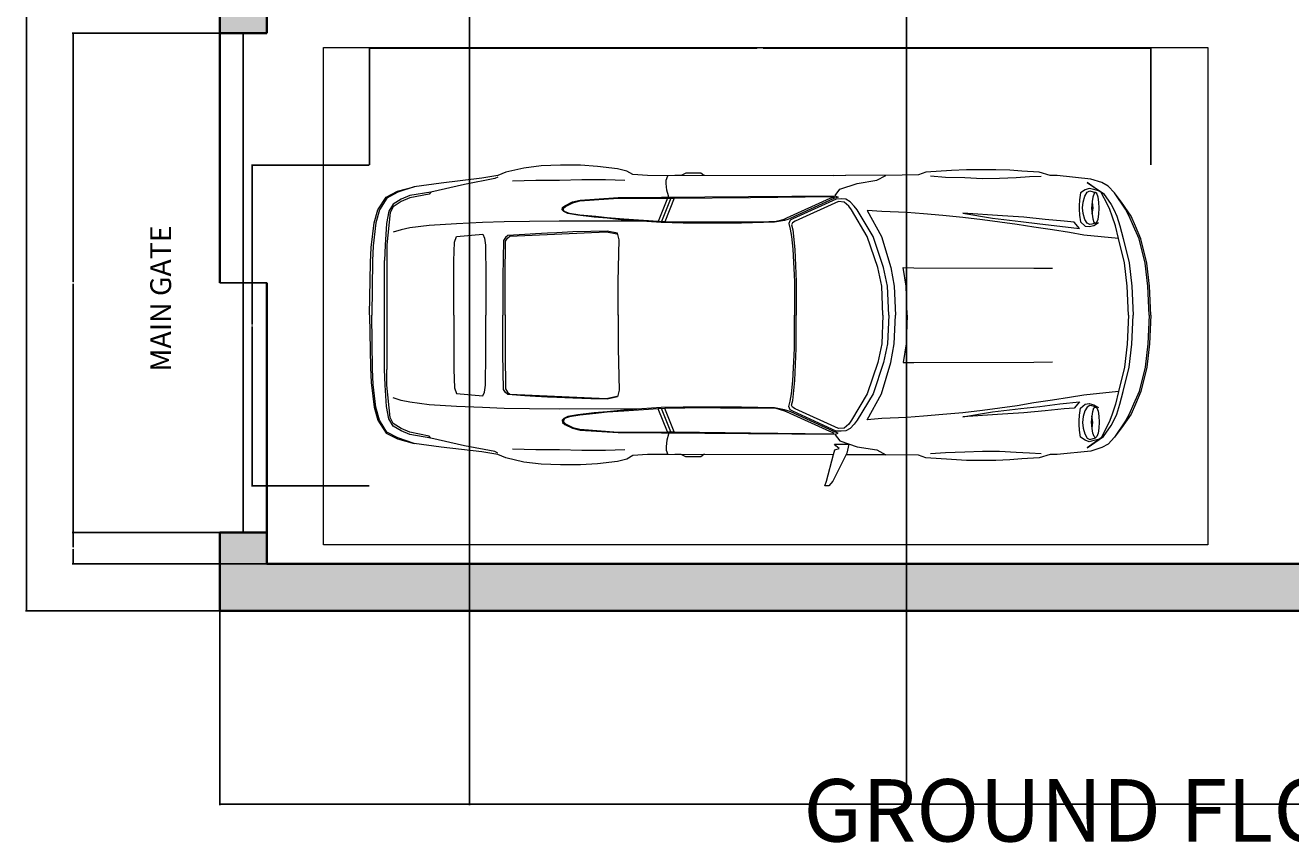
# Model space of a CAD drawing. Units: inches. Extents: x 2701 to 6846, y 811 to 2447.
# Tile 1 of 20: x 2701 to 2944, y 811 to 969. Entities that reach past the tile are written whole.
import ezdxf

# ---------------------------------------------------------------- set-up
doc = ezdxf.new("R2010")
doc.units = ezdxf.units.IN
for name, color, linetype, lineweight in [('A-ANNO-DIMS', 2, 'Continuous', 18), ('A-ANNO-TEXT', 7, 'Continuous', 18), ('A-ANNO-TITL', 7, 'Continuous', 35), ('C-PKNG', 8, 'Continuous', 18), ('C-PKNG-VEHI', 8, 'Continuous', 13), ('C-PROP', 7, 'Continuous', 35), ('C-SITE-GATE', 3, 'Continuous', 25)]:
    doc.layers.add(name, color=color, linetype=linetype, lineweight=lineweight)
doc.layers.add('C-PROP-PATT', color=18, linetype='Continuous', lineweight=13, true_color=0x000000)
doc.styles.get("Standard").update_dxf_attribs({"font": 'arial.ttf'})
doc.dimstyles.get("Standard").update_dxf_attribs({"dimtxt": 0.18, "dimasz": 0.18, "dimexe": 0.18, "dimexo": 0.0625, "dimgap": 0.09, "dimtad": 0, "dimtih": 1, "dimtoh": 1, "dimdec": 4, "dimzin": 0, "dimdsep": 46, "dimtxsty": 'Standard', "dimcen": 0.09, "dimadec": 0, "dimazin": 0, "dimtfac": 1, "dimtdec": 4, "dimtofl": 0, "dimtmove": 0, "dimatfit": 3, "dimfxl": 1, "dimtolj": 1, "dimtzin": 0, "dimarcsym": 0})

# ---------------------------------------------------------------- blocks, each defined once
blk = doc.blocks.new('A$C7AB76BE8')
for p, q in [((1739.9, 1727), (1762, 1752)), ((1762, 1752), (1784, 1752)), ((1784, 1752), (1774.5, 1727)), ((1663.9, 1575), (1739.9, 1727)), ((1774.5, 1727), (1736.1, 1582.3)), ((550.5, 1581.5), (610.5, 1600.1)), ((610.5, 1600.1), (705.5, 1605.7)), ((705.5, 1605.7), (772, 1610.8)), ((772, 1610.8), (847.5, 1613.9)), ((847.5, 1613.9), (920.5, 1613.9)), ((920.5, 1613.9), (1009, 1613.9)), ((1009, 1613.9), (1091.5, 1608.7)), ((1091.5, 1608.7), (1230.5, 1600.1)), ((1230.5, 1600.1), (1271.9, 1585.4)), ((2445.4, 1581.9), (2461.4, 1594.4)), ((2461.4, 1594.4), (2543.4, 1594.4)), ((2543.4, 1594.4), (2568.9, 1581.9)), ((2834.4, 1587.5), (2866.4, 1606.5)), ((2866.4, 1606.5), (2916.9, 1619)), ((2916.9, 1619), (3027.4, 1632)), ((3027.4, 1632), (3119.4, 1638)), ((3119.4, 1638), (3229.9, 1638)), ((3229.9, 1638), (3334.4, 1635)), ((3334.4, 1635), (3429.4, 1622.5)), ((3429.4, 1622.5), (3527.4, 1600.5)), ((3527.4, 1600.5), (3571.8, 1582.3)), ((199, 1486.5), (234, 1524.5)), ((234, 1524.5), (268.5, 1543.5)), ((348.4, 1544.8), (259, 1483.9)), ((268.5, 1543.5), (329, 1562.5)), ((272, 1489.5), (348.4, 1544.8)), ((329, 1562.5), (512.5, 1581.5)), ((512.5, 1581.5), (550.5, 1581.5)), ((601, 1577.2), (664, 1574.1)), ((664, 1574.1), (737, 1569.8)), ((737, 1569.8), (828.5, 1565.5)), ((828.5, 1565.5), (920.5, 1564.6)), ((920.5, 1564.6), (1017.2, 1569)), ((1017.2, 1569), (1123, 1572)), ((1123, 1572), (1206.3, 1578)), ((1271.9, 1585.4), (1448.9, 1582.8)), ((1448.9, 1582.8), (1667.8, 1583.2)), ((1499.5, 1556), (1448.9, 1582.8)), ((1607, 1539.2), (1499.5, 1556)), ((1701.9, 1507.2), (1607, 1539.2)), ((1651.4, 1524.5), (1663.9, 1575)), ((1730.4, 1524.5), (1651.4, 1524.5)), ((1729.6, 1556), (1705, 1549.5)), ((1705, 1549.5), (1723.5, 1534.4)), ((1723.5, 1534.4), (1730.4, 1524.5)), ((1736.1, 1582.3), (1729.6, 1556)), ((1736.1, 1582.8), (2641.4, 1581.1)), ((2438.9, 1581.9), (2445.4, 1581.9)), ((2568.9, 1581.9), (2603.4, 1581.9)), ((2641.4, 1581.1), (2753.2, 1581.5)), ((2650.9, 1557.3), (2641.4, 1581.1)), ((2647.9, 1502.5), (2650.9, 1537.9)), ((2650.9, 1537.9), (2650.9, 1557.3)), ((2753.2, 1581.5), (2834.4, 1587.5)), ((2878, 1555.4), (2982.5, 1558.8)), ((2982.5, 1558.8), (3112, 1558.8)), ((3112, 1558.8), (3235.5, 1555.4)), ((3235.5, 1555.4), (3363.3, 1555.4)), ((3363.3, 1555.4), (3491.5, 1551.9)), ((3571.8, 1582.3), (3660.3, 1566.8)), ((3571.8, 1573.7), (3587.4, 1565.1)), ((3587.4, 1565.1), (3754, 1533.6)), ((3660.3, 1566.8), (3881.8, 1540.9)), ((3754, 1533.6), (3938.8, 1491.7)), ((3881.8, 1540.9), (4030.3, 1521)), ((139, 1398), (199, 1486.5)), ((161, 1435.6), (199, 1486.5)), ((259, 1483.9), (218, 1423.5)), ((237, 1423.5), (272, 1489.5)), ((284.1, 1436.9), (288.8, 1464.5)), ((287.5, 1499), (313, 1505.5)), ((288.8, 1464.5), (295.3, 1483)), ((295.3, 1483), (303.5, 1489.5)), ((333.3, 1498.6), (303.5, 1489.5)), ((303.5, 1489.5), (310.9, 1483)), ((310.9, 1483), (317.8, 1464.5)), ((313, 1505.5), (338.5, 1511.5)), ((317.8, 1464.5), (322.1, 1439.4)), ((349.3, 1491.3), (333.3, 1498.6)), ((338.5, 1511.5), (359.6, 1503.8)), ((361.8, 1469.2), (349.3, 1491.3)), ((359.6, 1503.8), (384.7, 1486.5)), ((370.4, 1437.3), (361.8, 1469.2)), ((384.7, 1486.5), (391.2, 1448.5)), ((1668.7, 1452), (1693.7, 1454.1)), ((1693.7, 1454.1), (1720.9, 1453.3)), ((1727.4, 1473.1), (1701.9, 1507.2)), ((1727.4, 1470.5), (1709.7, 1464.1)), ((1709.7, 1464.1), (1734.3, 1455.8)), ((2913.9, 1461.5), (1727.4, 1470.5)), ((1741.2, 1467.5), (1731.7, 1464.1)), ((1731.7, 1464.1), (1756.8, 1455.8)), ((1734.3, 1455.8), (1970.1, 1348.3)), ((2189.8, 1462.8), (1741.2, 1467.5)), ((1756.8, 1455.8), (1992.5, 1348.3)), ((2606.9, 1458), (2189.8, 1462.8)), ((2638.4, 1458), (2606.9, 1458)), ((2606.9, 1458), (2658.3, 1329.8)), ((2625.4, 1458), (2676.8, 1330.6)), ((2638.4, 1470.5), (2647.9, 1502.5)), ((2638.4, 1458), (2638.4, 1470.5)), ((2913.9, 1458.4), (2638.4, 1458)), ((2644, 1458), (2695, 1331.5)), ((3122.4, 1447.6), (2913.9, 1461.5)), ((3122.8, 1443.8), (2913.9, 1458.4)), ((3938.8, 1491.7), (4052.8, 1472.3)), ((3938.8, 1491.7), (3948.3, 1480.9)), ((3948.3, 1480.9), (4052.8, 1459.3)), ((4120.8, 1496.3), (4030.3, 1521)), ((4030.3, 1521), (4118.9, 1490.4)), ((4052.8, 1472.3), (4099.9, 1452.8)), ((4052.8, 1459.3), (4099.9, 1439.9)), ((4118.9, 1490.4), (4178.4, 1458.4)), ((4182.3, 1464.5), (4120.8, 1496.3)), ((4178.4, 1458.4), (4219, 1394.5)), ((4228.5, 1394.5), (4182.3, 1464.5)), ((108.8, 1360), (161, 1435.6)), ((118.3, 1360), (139, 1398)), ((202.1, 1395.4), (186.5, 1360.4)), ((218, 1423.5), (202.1, 1395.4)), ((211.6, 1360.4), (224.5, 1395.4)), ((224.5, 1395.4), (237, 1423.5)), ((282.8, 1404), (284.1, 1436.9)), ((284.1, 1371.7), (282.8, 1404)), ((321.2, 1436.9), (316.9, 1404)), ((316.9, 1404), (322.5, 1372.1)), ((324.2, 1404), (321.2, 1371.7)), ((322.1, 1439.4), (324.2, 1404)), ((373.5, 1405.8), (370.4, 1437.3)), ((370.4, 1374.2), (373.5, 1405.8)), ((391.2, 1448.5), (392.5, 1417)), ((392.5, 1398), (391.2, 1366)), ((392.5, 1417), (392.5, 1398)), ((1335, 1379), (1471.8, 1385)), ((1471.8, 1385), (1551.7, 1391.5)), ((1551.7, 1391.5), (1473.1, 1249.5)), ((1519.3, 1249.5), (1607, 1394.5)), ((1551.3, 1249.5), (1637.6, 1394.5)), ((1607, 1394.5), (1622.1, 1415.3)), ((1622.1, 1415.3), (1645, 1439)), ((1637.6, 1394.5), (1651.4, 1415.3)), ((1645, 1439), (1668.7, 1452)), ((1651.4, 1415.3), (1676.9, 1437.3)), ((1676.9, 1437.3), (1709.3, 1439.4)), ((1709.3, 1439.4), (1946.3, 1331.9)), ((1720.9, 1453.3), (1959.3, 1344.9)), ((3163, 1437.7), (3122.4, 1447.6)), ((3161.2, 1433), (3122.8, 1443.8)), ((3201.8, 1413.1), (3161.2, 1433)), ((3206.1, 1416.6), (3163, 1437.7)), ((3179.8, 1375.1), (3207, 1385)), ((3189, 1373.7), (3211.8, 1385)), ((3213.1, 1403.6), (3201.8, 1413.1)), ((3219.1, 1406.6), (3206.1, 1416.6)), ((3207, 1385), (3213.5, 1393.2)), ((3211.8, 1385), (3220.4, 1393.7)), ((3213.5, 1393.2), (3213.1, 1403.6)), ((3220.4, 1393.7), (3219.1, 1406.6)), ((4099.9, 1452.8), (4144.3, 1426.1)), ((4099.9, 1439.9), (4144.3, 1411.4)), ((4144.3, 1426.1), (4168.1, 1386.8)), ((4144.3, 1411.4), (4160.3, 1379)), ((4168.1, 1386.8), (4180.2, 1319.8)), ((4219, 1394.5), (4238.9, 1322.9)), ((4248.4, 1322.9), (4228.5, 1394.5)), ((85.1, 1306), (108.8, 1360)), ((94.6, 1306), (118.3, 1360)), ((186.5, 1360.4), (169.2, 1306.5)), ((194.3, 1306.5), (211.6, 1360.4)), ((288.8, 1343.6), (284.1, 1371.7)), ((313, 1309.1), (287.5, 1325)), ((295.3, 1326.3), (288.8, 1343.6)), ((303.5, 1320.7), (295.3, 1326.3)), ((311.3, 1326.8), (303.5, 1320.7)), ((303.5, 1320.7), (323.8, 1315.5)), ((318.2, 1345.8), (311.3, 1326.8)), ((321.2, 1371.7), (318.2, 1345.8)), ((323.8, 1315.5), (333.3, 1313.8)), ((333.3, 1313.8), (349.3, 1322)), ((349.3, 1322), (361.8, 1342.3)), ((384.7, 1328.1), (359.6, 1305.6)), ((361.8, 1342.3), (370.4, 1374.2)), ((391.2, 1366), (384.7, 1328.1)), ((390.3, 1293.1), (418.8, 1327.6)), ((418.8, 1327.6), (474.9, 1332.4)), ((474.9, 1332.4), (577.7, 1342.3)), ((607, 1318.1), (498.7, 1304.3)), ((577.7, 1342.3), (695.1, 1353.5)), ((711.9, 1330.6), (607, 1318.1)), ((695.1, 1353.5), (812.5, 1361.7)), ((866.5, 1348.8), (711.9, 1330.6)), ((731.4, 1314.7), (920.5, 1340.1)), ((812.5, 1361.7), (1028, 1376)), ((1028, 1376), (866.5, 1348.8)), ((920.5, 1340.1), (1028, 1352.7)), ((1028, 1352.7), (1138.9, 1363)), ((1138.9, 1363), (1243, 1372.5)), ((1243, 1372.5), (1335, 1379)), ((1946.3, 1331.9), (1960.6, 1323.3)), ((1959.3, 1344.9), (1973.5, 1337.5)), ((1960.6, 1323.3), (1966.2, 1311.6)), ((1970.1, 1348.3), (1986, 1342.3)), ((1973.5, 1337.5), (1979.6, 1319)), ((1979.6, 1319), (1973.5, 1289.2)), ((1986, 1342.3), (2003.3, 1336.3)), ((1992.5, 1348.3), (2008.5, 1342.3)), ((2003.3, 1336.3), (2058.1, 1326.3)), ((2008.5, 1342.3), (2025.8, 1336.3)), ((2025.8, 1336.3), (2049.1, 1330.2)), ((2049.1, 1330.2), (2130.7, 1327.6)), ((2058.1, 1326.3), (2239.9, 1322)), ((2130.7, 1327.6), (2239.5, 1327.6)), ((2239.5, 1327.6), (2354.7, 1327.2)), ((2239.9, 1322), (2438.9, 1322)), ((2354.7, 1327.2), (2439.4, 1326.3)), ((2438.9, 1322), (2558.1, 1322)), ((2439.4, 1326.3), (2658.3, 1329.8)), ((2558.1, 1322), (2679, 1325.2)), ((2658.3, 1329.8), (2695.4, 1331.5)), ((2679, 1325.2), (2783.9, 1332.4)), ((2695.4, 1331.5), (2881.9, 1344)), ((2783.9, 1332.4), (2881.9, 1338.8)), ((2783.9, 1332.4), (3236.4, 1333.2)), ((2881.9, 1344), (2973.9, 1350.5)), ((2881.9, 1338.8), (2973.2, 1348.1)), ((2973.2, 1348.1), (3044.4, 1354.2)), ((2973.9, 1350.5), (3036, 1357.4)), ((3036, 1357.4), (3123.2, 1366)), ((3044.4, 1354.2), (3135.1, 1364.6)), ((3123.2, 1366), (3179.8, 1375.1)), ((3135.1, 1364.6), (3189, 1373.7)), ((3236.4, 1333.2), (3397.8, 1331.5)), ((3397.8, 1331.5), (3536.9, 1329.8)), ((3536.9, 1329.8), (3655.2, 1324.6)), ((3655.2, 1324.6), (3797.2, 1318.1)), ((3797.2, 1318.1), (3948.3, 1309.5)), ((4160.3, 1379), (4178.3, 1202.8)), ((4180.2, 1319.8), (4187.9, 1201.5)), ((4238.9, 1322.9), (4254.4, 1198.1)), ((4264.8, 1188.6), (4248.4, 1322.9)), ((55.3, 1236.5), (85.1, 1306)), ((64.8, 1236.5), (94.6, 1306)), ((169.2, 1306.5), (151.5, 1237)), ((177, 1237), (194.3, 1306.5)), ((177, 1237), (366.1, 1256.8)), ((338.5, 1303), (313, 1309.1)), ((359.6, 1305.6), (338.5, 1303)), ((366.1, 1256.8), (444.3, 1269.8)), ((498.7, 1304.3), (390.3, 1293.1)), ((444.3, 1269.8), (538, 1284.4)), ((538, 1284.4), (639.8, 1299.6)), ((639.8, 1299.6), (731.4, 1314.7)), ((1473.1, 1249.5), (1422.6, 1078.5)), ((1462.3, 1078.5), (1519.3, 1249.5)), ((1494.3, 1078.5), (1551.3, 1249.5)), ((1958.8, 1285.7), (1947.6, 1177.4)), ((1965.7, 1249.5), (1957.5, 1179.5)), ((1966.2, 1311.6), (1958.8, 1285.7)), ((1973.5, 1289.2), (1965.7, 1249.5)), ((2907.4, 1230.5), (2916.9, 1266.7)), ((2916.9, 1266.7), (2973.4, 1278.4)), ((2977.8, 1274.9), (2921.2, 1263.3)), ((2973.4, 1278.4), (3064.1, 1276.7)), ((3505.8, 1250.8), (2977.8, 1274.9)), ((3064.1, 1276.7), (3162.5, 1273.7)), ((3162.5, 1273.7), (3249.8, 1269.3)), ((3249.8, 1269.3), (3300.3, 1267.6)), ((3300.3, 1267.6), (3365.5, 1263.7)), ((3365.5, 1263.7), (3423.3, 1260.3)), ((3423.3, 1260.3), (3516.6, 1254.2)), ((3519.2, 1240), (3505.8, 1250.8)), ((3516.6, 1254.2), (3530, 1243)), ((3654.7, 1260.7), (3645.2, 1240.4)), ((3797.6, 1248.2), (3654.7, 1260.7)), ((3809.7, 1217.5), (3797.6, 1248.2)), ((3948.3, 1309.5), (4052.8, 1296.1)), ((4052.8, 1296.1), (4099.9, 1285.3)), ((4099.9, 1285.3), (4144.3, 1272.4)), ((22, 1103.5), (55.3, 1236.5)), ((31.5, 1103.5), (64.8, 1236.5)), ((151.5, 1237), (118.3, 1104)), ((143.8, 1104), (177, 1237)), ((1947.6, 1177.4), (1940.7, 1002.1)), ((1957.5, 1179.5), (1948.5, 1002.1)), ((2913.4, 1002.5), (2907.4, 1230.5)), ((3529.1, 1222.7), (3519.2, 1240)), ((3531.2, 1027.6), (3529.1, 1222.7)), ((3530, 1243), (3540.3, 1226.2)), ((3540.3, 1226.2), (3543.8, 1030.6)), ((3638.8, 1202), (3637.9, 1030.6)), ((3645.2, 1240.4), (3638.8, 1202)), ((3813.2, 1116.1), (3809.7, 1217.5)), ((4178.3, 1202.8), (4179.5, 1117.3)), ((4187.9, 1201.5), (4191, 1116.5)), ((4254.4, 1198.1), (4257.9, 1115.6)), ((4268.2, 1106.1), (4264.8, 1188.6)), ((3813.2, 819), (3813.2, 1116.1)), ((4179.5, 520.7), (4179.5, 1117.3)), ((4191, 1116.5), (4191, 521.5)), ((4257.9, 1115.6), (4261.3, 819)), ((7.8, 977), (22, 1103.5)), ((17.3, 977), (31.5, 1103.5)), ((118.3, 1104), (104.1, 977.5)), ((129.5, 977.5), (143.8, 1104)), ((639.8, 1075.9), (538, 1074.6)), ((1296.5, 1078.1), (639.8, 1075.9)), ((1354.4, 1078.5), (1296.5, 1078.1)), ((1338.8, 977), (1354.4, 1078.5)), ((1422.6, 1078.5), (1403.6, 977)), ((1440.3, 977), (1462.3, 1078.5)), ((1472.3, 977), (1494.3, 1078.5)), ((4273.9, 819.5), (4268.2, 1106.1)), ((0, 819), (7.8, 977)), ((9.1, 819), (17.3, 977)), ((104.1, 977.5), (96.3, 819)), ((121.8, 819), (129.5, 977.5)), ((1332.4, 819), (1338.8, 977)), ((1403.6, 977), (1397.1, 819)), ((1433.8, 819), (1440.3, 977)), ((1465.8, 819), (1472.3, 977)), ((1940.7, 1002.1), (1939.4, 819)), ((1948.5, 1002.1), (1949.3, 819)), ((2913.9, 818.6), (2913.4, 1002.5)), ((3531.2, 818.6), (3531.2, 1027.6)), ((3543.8, 1030.6), (3543.8, 819)), ((3637.9, 1030.6), (3637.9, 819)), ((0, 819), (7.8, 661)), ((9.1, 819), (17.3, 661)), ((104.1, 660.6), (96.3, 819)), ((121.8, 819), (129.5, 660.6)), ((1332.4, 819), (1338.8, 661)), ((1403.6, 661), (1397.1, 819)), ((1433.8, 819), (1440.3, 661)), ((1465.8, 819), (1472.3, 661)), ((1940.7, 636), (1939.4, 819)), ((1948.5, 636), (1949.3, 819)), ((2913.9, 819.5), (2913.4, 635.5)), ((3531.2, 819.5), (3531.2, 610.5)), ((3543.8, 607.5), (3543.8, 819)), ((3637.9, 607.5), (3637.9, 819)), ((3813.2, 819), (3813.2, 522)), ((4257.9, 522.4), (4261.3, 819)), ((4273.9, 818.6), (4268.2, 531.9)), ((7.8, 661), (22, 534.5)), ((17.3, 661), (31.5, 534.5)), ((118.3, 534.1), (104.1, 660.6)), ((129.5, 660.6), (143.8, 534.1)), ((1338.8, 661), (1354.4, 559.5)), ((1422.6, 559.5), (1403.6, 661)), ((1440.3, 661), (1462.3, 559.5)), ((1472.3, 661), (1494.3, 559.5)), ((1947.6, 460.7), (1940.7, 636)), ((1957.5, 458.5), (1948.5, 636)), ((2913.4, 635.5), (2907.4, 407.6)), ((639.8, 562.1), (538, 563.4)), ((1296.5, 560), (639.8, 562.1)), ((1354.4, 559.5), (1296.5, 560)), ((1473.1, 388.6), (1422.6, 559.5)), ((1462.3, 559.5), (1519.3, 388.6)), ((1494.3, 559.5), (1551.3, 388.6)), ((3531.2, 610.5), (3529.1, 415.3)), ((3540.3, 411.9), (3543.8, 607.5)), ((3638.8, 436.1), (3637.9, 607.5)), ((22, 534.5), (55.3, 401.5)), ((31.5, 534.5), (64.8, 401.5)), ((151.5, 401.1), (118.3, 534.1)), ((143.8, 534.1), (177, 401.1)), ((3813.2, 522), (3809.7, 420.5)), ((4178.3, 435.3), (4179.5, 520.7)), ((4187.9, 436.5), (4191, 521.5)), ((4254.4, 439.9), (4257.9, 522.4)), ((4268.2, 531.9), (4264.8, 449.4)), ((1958.8, 352.3), (1947.6, 460.7)), ((1965.7, 388.6), (1957.5, 458.5)), ((3529.1, 415.3), (3519.2, 398.1)), ((3645.2, 397.6), (3638.8, 436.1)), ((3809.7, 420.5), (3797.6, 389.9)), ((4160.3, 259), (4178.3, 435.3)), ((4180.2, 318.2), (4187.9, 436.5)), ((4238.9, 315.2), (4254.4, 439.9)), ((4264.8, 449.4), (4248.4, 315.2)), ((55.3, 401.5), (85.1, 332)), ((64.8, 401.5), (94.6, 332)), ((169.2, 331.6), (151.5, 401.1)), ((177, 401.1), (194.3, 331.6)), ((177, 401.1), (366.1, 381.2)), ((366.1, 381.2), (444.3, 368.3)), ((444.3, 368.3), (538, 353.6)), ((538, 353.6), (639.8, 338.5)), ((1551.7, 246.5), (1473.1, 388.6)), ((1519.3, 388.6), (1607, 243.5)), ((1551.3, 388.6), (1637.6, 243.5)), ((1966.2, 326.4), (1958.8, 352.3)), ((1973.5, 348.9), (1965.7, 388.6)), ((1979.6, 319.1), (1973.5, 348.9)), ((2907.4, 407.6), (2916.9, 371.3)), ((2916.9, 371.3), (2973.4, 359.6)), ((2977.8, 363.1), (2921.2, 374.8)), ((2973.4, 359.6), (3064.1, 361.4)), ((3505.8, 387.3), (2977.8, 363.1)), ((3064.1, 361.4), (3162.5, 364.4)), ((3162.5, 364.4), (3249.8, 368.7)), ((3249.8, 368.7), (3300.3, 370.4)), ((3300.3, 370.4), (3365.5, 374.3)), ((3365.5, 374.3), (3423.3, 377.8)), ((3423.3, 377.8), (3516.6, 383.8)), ((3519.2, 398.1), (3505.8, 387.3)), ((3516.6, 383.8), (3530, 395)), ((3530, 395), (3540.3, 411.9)), ((3654.7, 377.3), (3645.2, 397.6)), ((3797.6, 389.9), (3654.7, 377.3)), ((4052.8, 341.9), (4099.9, 352.7)), ((4099.9, 352.7), (4144.3, 365.7)), ((85.1, 332), (108.8, 278)), ((94.6, 332), (118.3, 278)), ((108.8, 278), (161, 202.5)), ((118.3, 278), (139, 240.1)), ((186.5, 277.6), (169.2, 331.6)), ((202.1, 242.6), (186.5, 277.6)), ((194.3, 331.6), (211.6, 277.6)), ((211.6, 277.6), (224.5, 242.6)), ((288.8, 294.5), (284.1, 266.4)), ((313, 329), (287.5, 313)), ((295.3, 311.7), (288.8, 294.5)), ((303.5, 317.3), (295.3, 311.7)), ((303.5, 317.3), (323.8, 322.5)), ((311.3, 311.3), (303.5, 317.3)), ((318.2, 292.3), (311.3, 311.3)), ((338.5, 335), (313, 329)), ((321.2, 266.4), (318.2, 292.3)), ((323.8, 322.5), (333.3, 324.2)), ((333.3, 324.2), (349.3, 316)), ((359.6, 332.4), (338.5, 335)), ((349.3, 316), (361.8, 295.7)), ((384.7, 310), (359.6, 332.4)), ((361.8, 295.7), (370.4, 263.8)), ((391.2, 272), (384.7, 310)), ((390.3, 345), (418.8, 310.4)), ((498.7, 333.7), (390.3, 345)), ((418.8, 310.4), (474.9, 305.7)), ((474.9, 305.7), (577.7, 295.7)), ((607, 319.9), (498.7, 333.7)), ((577.7, 295.7), (695.1, 284.5)), ((711.9, 307.4), (607, 319.9)), ((639.8, 338.5), (731.4, 323.4)), ((695.1, 284.5), (812.5, 276.3)), ((866.5, 289.3), (711.9, 307.4)), ((731.4, 323.4), (920.5, 297.9)), ((1028, 262.1), (866.5, 289.3)), ((920.5, 297.9), (1028, 285.4)), ((1028, 285.4), (1138.9, 275)), ((1709.3, 198.6), (1946.3, 306.1)), ((1720.9, 184.8), (1959.3, 293.2)), ((1734.3, 182.2), (1970.1, 289.7)), ((1756.8, 182.2), (1992.5, 289.7)), ((1946.3, 306.1), (1960.6, 314.7)), ((1959.3, 293.2), (1973.5, 300.5)), ((1960.6, 314.7), (1966.2, 326.4)), ((1970.1, 289.7), (1986, 295.7)), ((1973.5, 300.5), (1979.6, 319.1)), ((1986, 295.7), (2003.3, 301.8)), ((1992.5, 289.7), (2008.5, 295.7)), ((2003.3, 301.8), (2058.1, 311.7)), ((2008.5, 295.7), (2025.8, 301.8)), ((2025.8, 301.8), (2049.1, 307.8)), ((2049.1, 307.8), (2130.7, 310.4)), ((2058.1, 311.7), (2239.9, 316)), ((2130.7, 310.4), (2239.5, 310.4)), ((2239.5, 310.4), (2354.7, 310.9)), ((2239.9, 316), (2438.9, 316)), ((2354.7, 310.9), (2439.4, 311.7)), ((2438.9, 316), (2558.1, 316)), ((2439.4, 311.7), (2658.3, 308.3)), ((2558.1, 316), (2679, 312.8)), ((2606.9, 180), (2658.3, 308.3)), ((2625.4, 180), (2676.8, 307.4)), ((2644, 180), (2695, 306.5)), ((2658.3, 308.3), (2695.4, 306.5)), ((2679, 312.8), (2783.9, 305.7)), ((2695.4, 306.5), (2881.9, 294)), ((2783.9, 305.7), (3236.4, 304.8)), ((2783.9, 305.7), (2881.9, 299.2)), ((2881.9, 299.2), (2973.2, 290)), ((2881.9, 294), (2973.9, 287.5)), ((2973.2, 290), (3044.4, 283.9)), ((2973.9, 287.5), (3036, 280.6)), ((3036, 280.6), (3123.2, 272)), ((3044.4, 283.9), (3135.1, 273.4)), ((3236.4, 304.8), (3397.8, 306.5)), ((3397.8, 306.5), (3536.9, 308.3)), ((3536.9, 308.3), (3655.2, 313.4)), ((3655.2, 313.4), (3797.2, 319.9)), ((3797.2, 319.9), (3948.3, 328.6)), ((3948.3, 328.6), (4052.8, 341.9)), ((4168.1, 251.3), (4180.2, 318.2)), ((4219, 243.5), (4238.9, 315.2)), ((4248.4, 315.2), (4228.5, 243.5)), ((139, 240.1), (199, 151.5)), ((218, 214.6), (202.1, 242.6)), ((259, 154.1), (218, 214.6)), ((224.5, 242.6), (237, 214.6)), ((237, 214.6), (272, 148.5)), ((284.1, 266.4), (282.8, 234)), ((282.8, 234), (284.1, 201.2)), ((316.9, 234), (322.5, 266)), ((321.2, 201.2), (316.9, 234)), ((324.2, 234), (321.2, 266.4)), ((322.1, 198.6), (324.2, 234)), ((370.4, 263.8), (373.5, 232.3)), ((373.5, 232.3), (370.4, 200.8)), ((392.5, 240.1), (391.2, 272)), ((391.2, 189.5), (392.5, 221.1)), ((392.5, 221.1), (392.5, 240.1)), ((812.5, 276.3), (1028, 262.1)), ((1138.9, 275), (1243, 265.5)), ((1243, 265.5), (1335, 259)), ((1335, 259), (1471.8, 253)), ((1471.8, 253), (1551.7, 246.5)), ((1607, 243.5), (1622.1, 222.8)), ((1622.1, 222.8), (1645, 199)), ((1637.6, 243.5), (1651.4, 222.8)), ((1651.4, 222.8), (1676.9, 200.8)), ((3123.2, 272), (3179.8, 262.9)), ((3135.1, 273.4), (3189, 264.3)), ((3201.8, 224.9), (3161.2, 205.1)), ((3206.1, 221.5), (3163, 200.3)), ((3179.8, 262.9), (3207, 253)), ((3189, 264.3), (3211.8, 253)), ((3213.1, 234.4), (3201.8, 224.9)), ((3219.1, 231.4), (3206.1, 221.5)), ((3207, 253), (3213.5, 244.8)), ((3211.8, 253), (3220.4, 244.4)), ((3213.5, 244.8), (3213.1, 234.4)), ((3220.4, 244.4), (3219.1, 231.4)), ((4099.9, 198.2), (4144.3, 226.7)), ((4099.9, 185.2), (4144.3, 212)), ((4144.3, 226.7), (4160.3, 259)), ((4144.3, 212), (4168.1, 251.3)), ((4178.4, 179.6), (4219, 243.5)), ((4228.5, 243.5), (4182.3, 173.6)), ((161, 202.5), (199, 151.5)), ((199, 151.5), (234, 113.5)), ((348.4, 93.3), (259, 154.1)), ((272, 148.5), (348.4, 93.3)), ((284.1, 201.2), (288.8, 173.6)), ((287.5, 139), (313, 132.5)), ((288.8, 173.6), (295.3, 155)), ((295.3, 155), (303.5, 148.5)), ((303.5, 148.5), (310.9, 155)), ((333.3, 139.5), (303.5, 148.5)), ((310.9, 155), (317.8, 173.6)), ((317.8, 173.6), (322.1, 198.6)), ((349.3, 146.8), (333.3, 139.5)), ((361.8, 168.8), (349.3, 146.8)), ((359.6, 134.3), (384.7, 151.5)), ((370.4, 200.8), (361.8, 168.8)), ((384.7, 151.5), (391.2, 189.5)), ((1645, 199), (1668.7, 186.1)), ((1668.7, 186.1), (1693.7, 183.9)), ((1676.9, 200.8), (1709.3, 198.6)), ((1693.7, 183.9), (1720.9, 184.8)), ((1727.4, 164.9), (1701.9, 130.8)), ((1709.7, 174), (1734.3, 182.2)), ((1727.4, 167.5), (1709.7, 174)), ((2913.9, 176.6), (1727.4, 167.5)), ((1731.7, 174), (1756.8, 182.2)), ((1741.2, 170.5), (1731.7, 174)), ((2189.8, 175.3), (1741.2, 170.5)), ((2606.9, 180), (2189.8, 175.3)), ((2638.4, 180), (2606.9, 180)), ((2638.4, 180), (2638.4, 167.5)), ((2913.9, 179.6), (2638.4, 180)), ((2638.4, 167.5), (2647.9, 135.6)), ((3122.8, 194.3), (2913.9, 179.6)), ((3122.4, 190.4), (2913.9, 176.6)), ((3163, 200.3), (3122.4, 190.4)), ((3161.2, 205.1), (3122.8, 194.3)), ((3754, 104.5), (3938.8, 146.4)), ((3938.8, 146.4), (4052.8, 165.8)), ((3938.8, 146.4), (3948.3, 157.2)), ((3948.3, 157.2), (4052.8, 178.7)), ((4030.3, 117), (4118.9, 147.7)), ((4120.8, 141.8), (4030.3, 117)), ((4052.8, 178.7), (4099.9, 198.2)), ((4052.8, 165.8), (4099.9, 185.2)), ((4118.9, 147.7), (4178.4, 179.6)), ((4182.3, 173.6), (4120.8, 141.8)), ((234, 113.5), (268.5, 94.6)), ((268.5, 94.6), (329, 75.6)), ((313, 132.5), (338.5, 126.5)), ((329, 75.6), (512.5, 56.6)), ((338.5, 126.5), (359.6, 134.3)), ((737, 68.2), (828.5, 72.5)), ((828.5, 72.5), (920.5, 73.4)), ((920.5, 73.4), (1017.2, 69.1)), ((1499.5, 82), (1448.9, 55.3)), ((1607, 98.9), (1499.5, 82)), ((1701.9, 130.8), (1607, 98.9)), ((2650.9, 80.7), (2641.4, 57)), ((2647.9, 135.6), (2650.9, 100.2)), ((2650.9, 100.2), (2650.9, 80.7)), ((2878, 82.7), (2982.5, 79.2)), ((2982.5, 79.2), (3112, 79.2)), ((3112, 79.2), (3235.5, 82.7)), ((3235.5, 82.7), (3363.3, 82.7)), ((3363.3, 82.7), (3491.5, 86.1)), ((3571.8, 64.3), (3587.4, 73)), ((3571.8, 55.7), (3660.3, 71.2)), ((3587.4, 73), (3754, 104.5)), ((3660.3, 71.2), (3881.8, 97.1)), ((3881.8, 97.1), (4030.3, 117)), ((512.5, 56.6), (550.5, 56.6)), ((550.5, 56.6), (610.5, 38)), ((601, 60.9), (664, 63.9)), ((610.5, 38), (705.5, 32.4)), ((664, 63.9), (737, 68.2)), ((705.5, 32.4), (772, 27.2)), ((772, 27.2), (847.5, 24.2)), ((847.5, 24.2), (920.5, 24.2)), ((920.5, 24.2), (1009, 24.2)), ((1009, 24.2), (1091.5, 29.4)), ((1017.2, 69.1), (1123, 66.1)), ((1091.5, 29.4), (1230.5, 38)), ((1123, 66.1), (1206.3, 60)), ((1230.5, 38), (1271.9, 52.7)), ((1271.9, 52.7), (1448.9, 55.3)), ((1448.9, 55.3), (1667.8, 54.8)), ((1736.1, 55.3), (1667.8, 54.8)), ((1736.1, 55.3), (2641.4, 57)), ((2438.9, 56.1), (2445.4, 56.1)), ((2445.4, 56.1), (2461.4, 43.6)), ((2461.4, 43.6), (2543.4, 43.6)), ((2543.4, 43.6), (2568.9, 56.1)), ((2568.9, 56.1), (2603.4, 56.1)), ((2641.4, 57), (2753.2, 56.6)), ((2753.2, 56.6), (2834.4, 50.5)), ((2834.4, 50.5), (2866.4, 31.5)), ((2866.4, 31.5), (2916.9, 19)), ((2916.9, 19), (3027.4, 6)), ((3027.4, 6), (3119.4, 0)), ((3119.4, 0), (3229.9, 0)), ((3229.9, 0), (3334.4, 3)), ((3334.4, 3), (3429.4, 15.5)), ((3429.4, 15.5), (3527.4, 37.6)), ((3527.4, 37.6), (3571.8, 55.7))]:
    blk.add_line(p, q)
blk = doc.blocks.new('*D61')
at = {"layer": 'A-ANNO-DIMS', "color": 0, "lineweight": -2, "transparency": 16777216}
for p, q in [((2766.73, 941.71), (2766.73, 964.36)), ((2766.91, 964.18), (2841.25, 964.18)), ((2916.76, 964.18), (2842.42, 964.18)), ((2916.94, 941.71), (2916.94, 964.36))]:
    blk.add_line(p, q, dxfattribs=at)
at = {"layer": 'A-ANNO-DIMS', "color": 0, "transparency": 16777216}
for points in [[(2766.91, 964.21), (2766.91, 964.15), (2766.73, 964.18)], [(2916.76, 964.21), (2916.76, 964.15), (2916.94, 964.18)]]:
    blk.add_solid(points, dxfattribs=at)
at = {"layer": 'Defpoints', "color": 0, "transparency": 16777216}
for p in [(2766.73, 964.18), (2766.73, 941.65), (2916.94, 941.65)]:
    blk.add_point(p, dxfattribs=at)
at = {"layer": 'A-ANNO-DIMS', "color": 0, "transparency": 16777216, "insert": (2841.83, 964.18), "char_height": 0.18, "attachment_point": 5}
blk.add_mtext('\\A1;CAR 150', dxfattribs=at)
blk = doc.blocks.new('*D62')
at = {"layer": 'A-ANNO-DIMS', "color": 0, "lineweight": -2, "transparency": 16777216}
for p, q in [((2766.67, 941.65), (2744.02, 941.65)), ((2744.2, 941.47), (2744.2, 911.05)), ((2744.2, 880.25), (2744.2, 910.68)), ((2766.67, 880.07), (2744.02, 880.07))]:
    blk.add_line(p, q, dxfattribs=at)
at = {"layer": 'A-ANNO-DIMS', "color": 0, "transparency": 16777216}
for points in [[(2744.17, 941.47), (2744.23, 941.47), (2744.2, 941.65)], [(2744.17, 880.25), (2744.23, 880.25), (2744.2, 880.07)]]:
    blk.add_solid(points, dxfattribs=at)
at = {"layer": 'Defpoints', "color": 0, "transparency": 16777216}
for p in [(2766.73, 941.65), (2744.2, 880.07), (2766.73, 880.07)]:
    blk.add_point(p, dxfattribs=at)
at = {"layer": 'A-ANNO-DIMS', "color": 0, "transparency": 16777216, "insert": (2744.2, 910.86), "char_height": 0.18, "attachment_point": 5}
blk.add_mtext('\\A1;62', dxfattribs=at)
blk = doc.blocks.new('*D65')
at = {"layer": 'A-ANNO-DIMS', "color": 0, "lineweight": -2, "transparency": 16777216}
for p, q in [((2737.97, 855.99), (2737.97, 818.67)), ((3145.97, 855.99), (3145.97, 818.67)), ((2738.15, 818.85), (2941.68, 818.85)), ((3145.79, 818.85), (2942.26, 818.85))]:
    blk.add_line(p, q, dxfattribs=at)
at = {"layer": 'A-ANNO-DIMS', "color": 0, "transparency": 16777216}
for points in [[(2738.15, 818.88), (2738.15, 818.82), (2737.97, 818.85)], [(3145.79, 818.88), (3145.79, 818.82), (3145.97, 818.85)]]:
    blk.add_solid(points, dxfattribs=at)
at = {"layer": 'Defpoints', "color": 0, "transparency": 16777216}
for p in [(2737.97, 856.05), (3145.97, 856.05), (3145.97, 818.85)]:
    blk.add_point(p, dxfattribs=at)
at = {"layer": 'A-ANNO-DIMS', "color": 0, "transparency": 16777216, "insert": (2941.97, 818.85), "char_height": 0.18, "attachment_point": 5}
blk.add_mtext('\\A1;408', dxfattribs=at)
blk = doc.blocks.new('*D66')
at = {"layer": 'A-ANNO-DIMS', "color": 0, "lineweight": -2, "transparency": 16777216}
for p, q in [((2737.91, 1504.05), (2700.59, 1504.05)), ((2700.77, 1503.87), (2700.77, 1180.23)), ((2700.77, 856.23), (2700.77, 1179.87)), ((2737.91, 856.05), (2700.59, 856.05))]:
    blk.add_line(p, q, dxfattribs=at)
at = {"layer": 'A-ANNO-DIMS', "color": 0, "transparency": 16777216}
for points in [[(2700.74, 1503.87), (2700.8, 1503.87), (2700.77, 1504.05)], [(2700.74, 856.23), (2700.8, 856.23), (2700.77, 856.05)]]:
    blk.add_solid(points, dxfattribs=at)
at = {"layer": 'Defpoints', "color": 0, "transparency": 16777216}
for p in [(2700.77, 1504.05), (2737.97, 1504.05), (2737.97, 856.05)]:
    blk.add_point(p, dxfattribs=at)
at = {"layer": 'A-ANNO-DIMS', "color": 0, "transparency": 16777216, "insert": (2700.77, 1180.05), "char_height": 0.18, "attachment_point": 5}
blk.add_mtext('\\A1;648', dxfattribs=at)
blk = doc.blocks.new('*D74')
at = {"layer": 'A-ANNO-DIMS', "color": 0, "lineweight": -2, "transparency": 16777216}
for p, q in [((2785.97, 1035.99), (2785.97, 818.67)), ((2869.97, 1029.99), (2869.97, 818.67)), ((2786.15, 818.85), (2827.75, 818.85)), ((2869.79, 818.85), (2828.19, 818.85))]:
    blk.add_line(p, q, dxfattribs=at)
at = {"layer": 'A-ANNO-DIMS', "color": 0, "transparency": 16777216}
for points in [[(2786.15, 818.88), (2786.15, 818.82), (2785.97, 818.85)], [(2869.79, 818.88), (2869.79, 818.82), (2869.97, 818.85)]]:
    blk.add_solid(points, dxfattribs=at)
at = {"layer": 'Defpoints', "color": 0, "transparency": 16777216}
for p in [(2785.97, 1036.05), (2869.97, 1030.05), (2869.97, 818.85)]:
    blk.add_point(p, dxfattribs=at)
at = {"layer": 'A-ANNO-DIMS', "color": 0, "transparency": 16777216, "insert": (2827.97, 818.85), "char_height": 0.18, "attachment_point": 5}
blk.add_mtext('\\A1;84', dxfattribs=at)
blk = doc.blocks.new('*D76')
at = {"layer": 'A-ANNO-DIMS', "color": 0, "lineweight": -2, "transparency": 16777216}
for p, q in [((2746.91, 967.05), (2709.59, 967.05)), ((2709.77, 966.87), (2709.77, 919.23)), ((2709.77, 871.23), (2709.77, 918.87)), ((2746.91, 871.05), (2709.59, 871.05))]:
    blk.add_line(p, q, dxfattribs=at)
at = {"layer": 'A-ANNO-DIMS', "color": 0, "transparency": 16777216}
for points in [[(2709.74, 966.87), (2709.8, 966.87), (2709.77, 967.05)], [(2709.74, 871.23), (2709.8, 871.23), (2709.77, 871.05)]]:
    blk.add_solid(points, dxfattribs=at)
at = {"layer": 'Defpoints', "color": 0, "transparency": 16777216}
for p in [(2709.77, 967.05), (2746.97, 967.05), (2746.97, 871.05)]:
    blk.add_point(p, dxfattribs=at)
at = {"layer": 'A-ANNO-DIMS', "color": 0, "transparency": 16777216, "insert": (2709.77, 919.05), "char_height": 0.18, "attachment_point": 5}
blk.add_mtext('\\A1;96', dxfattribs=at)
blk = doc.blocks.new('*D77')
at = {"layer": 'A-ANNO-DIMS', "color": 0, "lineweight": -2, "transparency": 16777216}
for p, q in [((2746.91, 871.05), (2709.59, 871.05)), ((2709.77, 870.87), (2709.77, 868.23)), ((2709.77, 865.23), (2709.77, 867.87)), ((2746.91, 865.05), (2709.59, 865.05))]:
    blk.add_line(p, q, dxfattribs=at)
at = {"layer": 'A-ANNO-DIMS', "color": 0, "transparency": 16777216}
for points in [[(2709.74, 870.87), (2709.8, 870.87), (2709.77, 871.05)], [(2709.74, 865.23), (2709.8, 865.23), (2709.77, 865.05)]]:
    blk.add_solid(points, dxfattribs=at)
at = {"layer": 'Defpoints', "color": 0, "transparency": 16777216}
for p in [(2709.77, 871.05), (2746.97, 871.05), (2746.97, 865.05)]:
    blk.add_point(p, dxfattribs=at)
at = {"layer": 'A-ANNO-DIMS', "color": 0, "transparency": 16777216, "insert": (2709.77, 868.05), "char_height": 0.18, "attachment_point": 5}
blk.add_mtext('\\A1;6', dxfattribs=at)

msp = doc.modelspace()

# ---------------------------------------------------------------- hatches: boundary and pattern name
at = {"layer": 'C-PROP-PATT'}
h = msp.add_hatch(color=256, dxfattribs=at)
h.dxf.hatch_style = 1
h.paths.add_polyline_path([(3145.97, 1504.05), (2737.97, 1504.05), (2737.97, 967.05), (2746.97, 967.05), (2746.97, 1495.05), (3136.97, 1495.05), (3136.97, 865.05), (3130.97, 865.05), (3130.97, 856.05), (3145.97, 856.05)])
h.paths.add_polyline_path([(3070.97, 865.05), (2746.97, 865.05), (2746.97, 871.05), (2737.97, 871.05), (2737.97, 856.05), (3070.97, 856.05)], flags=17)

# ---------------------------------------------------------------- linework, layer by layer
at = {"layer": 'C-PKNG'}
msp.add_lwpolyline([(2757.89, 964.3), (2927.89, 964.3), (2927.89, 868.68), (2757.89, 868.68)], close=True, dxfattribs=at)
at = {"layer": 'C-PROP'}
for p, q in [((2737.97, 919.05), (2737.97, 1504.05)), ((2746.97, 967.05), (2746.97, 1495.05)), ((2746.97, 967.05), (2737.97, 967.05)), ((2746.97, 865.05), (2746.97, 919.05)), ((2737.97, 856.05), (2737.97, 871.05)), ((2746.97, 871.05), (2737.97, 871.05)), ((3070.97, 865.05), (2746.97, 865.05)), ((3100.97, 856.05), (2737.97, 856.05))]:
    msp.add_line(p, q, dxfattribs=at)
at = {"layer": 'C-SITE-GATE'}
for p, q in [((2742.47, 967.05), (2742.47, 871.05)), ((2742.47, 919.05), (2737.97, 919.05)), ((2742.47, 919.05), (2746.97, 919.05))]:
    msp.add_line(p, q, dxfattribs=at)

# ---------------------------------------------------------------- block references
at = {"layer": 'C-PKNG-VEHI', "xscale": 0.0351465449131131, "yscale": 0.0351465449131131, "zscale": 0.0351465449131131, "rotation": 180}
msp.add_blockref('A$C7AB76BE8', (2916.94, 941.65), dxfattribs=at)

# ---------------------------------------------------------------- texts
at = {"layer": 'A-ANNO-TEXT', "insert": (2724.59, 902), "char_height": 4, "attachment_point": 1, "rotation": 90}
msp.add_mtext_dynamic_manual_height_columns('{\\fTimes New Roman|b0|i0|c0|p18;MAIN GATE}', width=36.377, gutter_width=12.5, heights=[0], dxfattribs=at)
at = {"layer": 'A-ANNO-TITL', "insert": (2850.15, 823.68), "char_height": 12, "attachment_point": 1}
msp.add_mtext_dynamic_manual_height_columns('{\\fTimes New Roman|b0|i0|c0|p18;GROUND FLOOR PLAN}', width=192.9852, gutter_width=12.5, heights=[0], dxfattribs=at)

# ---------------------------------------------------------------- dimensions: what is measured, and where the dimension line sits
at = {"layer": 'A-ANNO-DIMS'}
for base, p1, p2, angle, picture, middle in [((2700.77, 1504.05), (2737.97, 856.05), (2737.97, 1504.05), 90, '*D66', (2700.77, 1180.05)), ((2709.77, 967.05), (2746.97, 871.05), (2746.97, 967.05), 90, '*D76', (2709.77, 919.05)), ((2744.2, 880.07), (2766.73, 941.65), (2766.73, 880.07), 270, '*D62', (2744.2, 910.86)), ((2709.77, 871.05), (2746.97, 865.05), (2746.97, 871.05), 90, '*D77', (2709.77, 868.05))]:
    dim = msp.add_linear_dim(base=base, p1=p1, p2=p2, angle=angle, dimstyle='Standard', override={"dimdec": 0, "dimlfac": 1, "dimrnd": 0, "dimzin": 0, "dimdsep": 46, "dimlunit": 2}, dxfattribs=at)
    dim.commit()
    dim.dimension.update_dxf_attribs({"geometry": picture, "text_midpoint": middle})
for base, p1, p2, picture, middle in [((2869.97, 818.85), (2785.97, 1036.05), (2869.97, 1030.05), '*D74', (2827.97, 818.85)), ((3145.97, 818.85), (2737.97, 856.05), (3145.97, 856.05), '*D65', (2941.97, 818.85))]:
    dim = msp.add_linear_dim(base=base, p1=p1, p2=p2, dimstyle='Standard', override={"dimdec": 0, "dimlfac": 1, "dimrnd": 0, "dimzin": 0, "dimdsep": 46, "dimlunit": 2}, dxfattribs=at)
    dim.commit()
    dim.dimension.update_dxf_attribs({"geometry": picture, "text_midpoint": middle})
dim = msp.add_linear_dim(base=(2766.73, 964.18), p1=(2916.94, 941.65), p2=(2766.73, 941.65), angle=180, text='CAR <>', dimstyle='Standard', override={"dimdec": 0, "dimlfac": 1, "dimrnd": 0, "dimzin": 0, "dimdsep": 46, "dimlunit": 2}, dxfattribs=at)
dim.commit()
dim.dimension.update_dxf_attribs({"geometry": '*D61', "text_midpoint": (2841.83, 964.18)})

doc.saveas('drawing.dxf')
